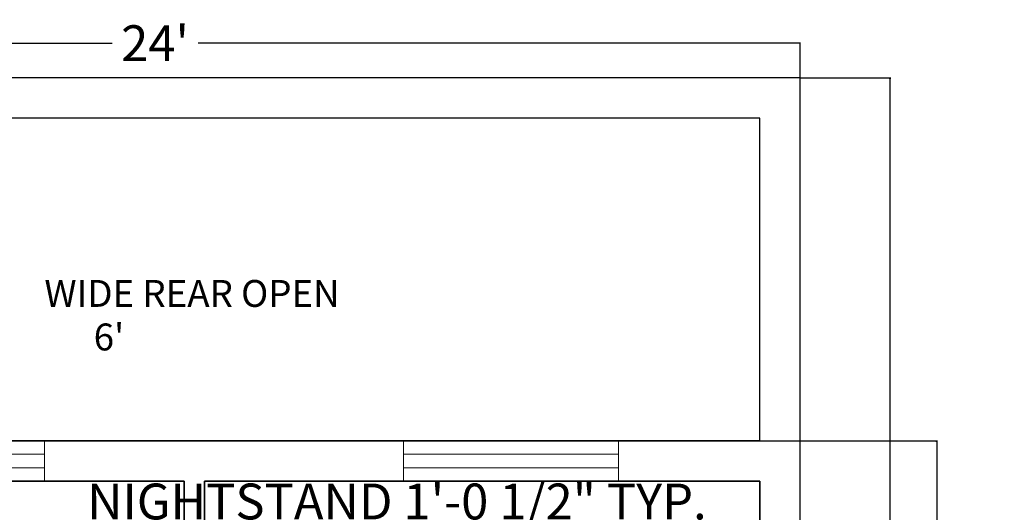
# Model space of a CAD drawing. Units: inches. Extents: x -11 to 443, y 65 to 743.
# Tile 10 of 10: x 158 to 378, y 610 to 720. Entities that reach past the tile are written whole.
import ezdxf

# ---------------------------------------------------------------- set-up
doc = ezdxf.new("R2010")
doc.units = ezdxf.units.IN
doc.header["$MEASUREMENT"] = 0
for name, color, linetype, lineweight in [('A-ANNO-DIMS', 2, 'Continuous', 18), ('A-AREA-IDEN', 2, 'Continuous', 18), ('A-GLAZ', 4, 'Continuous', 18), ('A-WALL', 7, 'Continuous', 35), ('A-WALL-SITE', 7, 'Continuous', 30), ('C-PROP', 3, 'Continuous', 30)]:
    doc.layers.add(name, color=color, linetype=linetype, lineweight=lineweight)
doc.styles.get("Standard").update_dxf_attribs({"font": 'italic8.shx'})
doc.dimstyles.get("Standard").update_dxf_attribs({"dimtxt": 8, "dimasz": 0.18, "dimexe": 0.18, "dimexo": 0.0625, "dimgap": 0.09, "dimtad": 0, "dimtih": 1, "dimtoh": 1, "dimzin": 0, "dimdsep": 46, "dimlunit": 3, "dimtxsty": 'Standard', "dimblk": 'CLOSEDBLANK', "dimcen": 0.09, "dimclrd": 6, "dimclre": 5, "dimclrt": 4, "dimadec": 0, "dimazin": 0, "dimtfac": 1, "dimtofl": 0, "dimtmove": 0, "dimatfit": 3, "dimfxl": 1, "dimtolj": 1, "dimtzin": 0, "dimarcsym": 0})

# ---------------------------------------------------------------- blocks, each defined once
blk = doc.blocks.new('_ClosedBlank')
at = {"color": 0, "linetype": 'ByBlock', "lineweight": -2}
for p, q in [((-1, 0.167), (0, 0)), ((-1, 0.167), (-1, -0.167)), ((0, 0), (-1, -0.167))]:
    blk.add_line(p, q, dxfattribs=at)
blk = doc.blocks.new('*D5')
at = {"layer": 'A-ANNO-DIMS', "color": 0, "lineweight": -2, "transparency": 16777216}
for p, q in [((44.21, 706.98), (44.21, 714.84)), ((44.39, 714.66), (178.6, 714.66)), ((332.03, 714.66), (197.82, 714.66)), ((332.21, 706.98), (332.21, 714.84))]:
    blk.add_line(p, q, dxfattribs=at)
at = {"layer": 'Defpoints', "color": 0, "lineweight": 100, "transparency": 16777216}
for p in [(332.21, 714.66), (44.21, 706.92), (332.21, 706.92)]:
    blk.add_point(p, dxfattribs=at)
at = {"layer": 'A-ANNO-DIMS', "color": 0, "lineweight": -2, "transparency": 16777216, "xscale": 0.18, "yscale": 0.18, "zscale": 0.18, "rotation": 180}
blk.add_blockref('_ClosedBlank', (44.21, 714.66), dxfattribs=at)
at = {"layer": 'A-ANNO-DIMS', "color": 0, "lineweight": -2, "transparency": 16777216, "xscale": 0.18, "yscale": 0.18, "zscale": 0.18}
blk.add_blockref('_ClosedBlank', (332.21, 714.66), dxfattribs=at)
at = {"layer": 'A-ANNO-DIMS', "color": 0, "transparency": 16777216, "insert": (188.21, 714.66), "char_height": 8, "attachment_point": 5}
blk.add_mtext("\\A1;24'", dxfattribs=at)
blk = doc.blocks.new('*D6')
at = {"layer": 'A-ANNO-DIMS', "color": 0, "lineweight": -2, "transparency": 16777216}
for p, q in [((332.27, 706.92), (352.4, 706.92)), ((352.22, 706.74), (352.22, 411.77)), ((352.22, 107.1), (352.22, 402.07)), ((332.27, 106.92), (352.4, 106.92))]:
    blk.add_line(p, q, dxfattribs=at)
at = {"layer": 'Defpoints', "color": 0, "lineweight": 100, "transparency": 16777216}
for p in [(332.21, 706.92), (332.21, 106.92), (352.22, 106.92)]:
    blk.add_point(p, dxfattribs=at)
at = {"layer": 'A-ANNO-DIMS', "color": 0, "lineweight": -2, "transparency": 16777216, "xscale": 0.18, "yscale": 0.18, "zscale": 0.18}
for p, rotation in [((352.22, 706.92), 90), ((352.22, 106.92), 270)]:
    blk.add_blockref('_ClosedBlank', p, dxfattribs=dict(at, rotation=rotation))
at = {"layer": 'A-ANNO-DIMS', "color": 0, "transparency": 16777216, "insert": (352.22, 406.92), "char_height": 8, "attachment_point": 5}
blk.add_mtext("\\A1;50'", dxfattribs=at)
blk = doc.blocks.new('WIN-48x9')
for p, q in [((0, 48), (0, 0)), ((9, 48), (0, 48)), ((3, 0), (3, 48)), ((6, 0), (6, 48)), ((9, 0), (9, 48)), ((0, 0), (9, 0))]:
    blk.add_line(p, q)
blk = doc.blocks.new('*D26')
at = {"layer": 'A-ANNO-DIMS', "color": 5, "lineweight": -2, "transparency": 16777216}
for p, q in [((133.01, 610.6), (133.01, 612.57)), ((145.34, 610.6), (145.34, 612.57))]:
    blk.add_line(p, q, dxfattribs=at)
at = {"layer": 'A-ANNO-DIMS', "color": 6, "lineweight": -2, "transparency": 16777216}
for p, q in [((133.19, 612.39), (145.16, 612.39)), ((145.34, 612.39), (145.52, 612.39))]:
    blk.add_line(p, q, dxfattribs=at)
at = {"layer": 'Defpoints', "color": 0, "lineweight": 100, "transparency": 16777216}
for p in [(145.34, 612.39), (133.01, 610.54), (145.34, 610.54)]:
    blk.add_point(p, dxfattribs=at)
at = {"layer": 'A-ANNO-DIMS', "color": 6, "lineweight": -2, "transparency": 16777216, "xscale": 0.18, "yscale": 0.18, "zscale": 0.18, "rotation": 180}
blk.add_blockref('_ClosedBlank', (133.01, 612.39), dxfattribs=at)
at = {"layer": 'A-ANNO-DIMS', "color": 6, "lineweight": -2, "transparency": 16777216, "xscale": 0.18, "yscale": 0.18, "zscale": 0.18}
blk.add_blockref('_ClosedBlank', (145.34, 612.39), dxfattribs=at)
at = {"layer": 'A-ANNO-DIMS', "color": 4, "transparency": 16777216, "insert": (242.18, 612.39), "char_height": 8, "attachment_point": 5}
blk.add_mtext('\\A1;NIGHTSTAND 1\'-0 1/2" TYP.', dxfattribs=at)
blk = doc.blocks.new('*D36')
at = {"layer": 'A-ANNO-DIMS', "color": 5, "lineweight": -2, "transparency": 16777216}
for p, q in [((323.27, 625.92), (362.85, 625.92)), ((323.27, 211.92), (362.85, 211.92))]:
    blk.add_line(p, q, dxfattribs=at)
at = {"layer": 'A-ANNO-DIMS', "color": 6, "lineweight": -2, "transparency": 16777216}
for p, q in [((362.67, 625.74), (362.67, 423.77)), ((362.67, 212.1), (362.67, 414.07))]:
    blk.add_line(p, q, dxfattribs=at)
at = {"layer": 'Defpoints', "color": 0, "lineweight": 100, "transparency": 16777216}
for p in [(323.21, 625.92), (362.67, 625.92), (323.21, 211.92)]:
    blk.add_point(p, dxfattribs=at)
at = {"layer": 'A-ANNO-DIMS', "color": 6, "lineweight": -2, "transparency": 16777216, "xscale": 0.18, "yscale": 0.18, "zscale": 0.18}
for p, rotation in [((362.67, 625.92), 90), ((362.67, 211.92), 270)]:
    blk.add_blockref('_ClosedBlank', p, dxfattribs=dict(at, rotation=rotation))
at = {"layer": 'A-ANNO-DIMS', "color": 4, "transparency": 16777216, "insert": (362.67, 418.92), "char_height": 8, "attachment_point": 5}
blk.add_mtext('\\A1;34\'-6"', dxfattribs=at)

msp = doc.modelspace()

# ---------------------------------------------------------------- linework, layer by layer
at = {"layer": 'A-WALL'}
for p, q in [((323.209, 625.92), (53.209, 625.92)), ((194.709, 616.92), (53.209, 616.92)), ((194.709, 616.92), (194.709, 522.42)), ((323.209, 616.92), (199.209, 616.92)), ((199.209, 616.92), (199.209, 522.42)), ((323.209, 522.42), (323.209, 616.92))]:
    msp.add_line(p, q, dxfattribs=at)
at = {"layer": 'A-WALL-SITE'}
for p, q in [((323.209, 697.92), (53.209, 697.92)), ((323.209, 625.92), (323.209, 697.92))]:
    msp.add_line(p, q, dxfattribs=at)
at = {"layer": 'C-PROP'}
msp.add_lwpolyline([(44.209, 106.92), (332.209, 106.92), (332.209, 706.92), (44.209, 706.92)], close=True, dxfattribs=at)

# ---------------------------------------------------------------- block references
at = {"layer": 'A-GLAZ', "rotation": 90.00000000000003}
for p in [(163.513, 616.92), (291.656, 616.92)]:
    msp.add_blockref('WIN-48x9', p, dxfattribs=at)

# ---------------------------------------------------------------- texts
at = {"layer": 'A-AREA-IDEN'}
for s, p in [('WIDE REAR OPEN', (163.503, 655.821)), ("      6'", (163.503, 646.107))]:
    msp.add_text(s, height=6, dxfattribs=at).set_placement(p)

# ---------------------------------------------------------------- dimensions: what is measured, and where the dimension line sits
at = {"layer": 'A-ANNO-DIMS'}
dim = msp.add_linear_dim(base=(332.209, 714.661), p1=(44.209, 706.92), p2=(332.209, 706.92), dimstyle='Standard', override={"dimclrd": 0, "dimclre": 0, "dimclrt": 0}, dxfattribs=at)
dim.commit()
dim.dimension.update_dxf_attribs({"geometry": '*D5', "text_midpoint": (188.209, 714.661)})
for base, p1, p2, override, picture, middle in [((352.221, 106.92), (332.209, 706.92), (332.209, 106.92), {"dimclrd": 0, "dimclre": 0, "dimclrt": 0}, '*D6', (352.221, 406.92)), ((362.669, 625.92), (323.209, 211.92), (323.209, 625.92), {"dimdec": 1, "dimlfac": 1, "dimrnd": 0, "dimzin": 1, "dimdsep": 46, "dimlunit": 4, "dimfrac": 2}, '*D36', (362.669, 418.92))]:
    dim = msp.add_linear_dim(base=base, p1=p1, p2=p2, angle=90, dimstyle='Standard', override=override, dxfattribs=at)
    dim.commit()
    dim.dimension.update_dxf_attribs({"geometry": picture, "text_midpoint": middle})
dim = msp.add_linear_dim(base=(145.337, 612.387), p1=(133.013, 610.539), p2=(145.337, 610.539), text='NIGHTSTAND <> TYP.', dimstyle='Standard', override={"dimdec": 1, "dimlfac": 1, "dimrnd": 0, "dimzin": 1, "dimdsep": 46, "dimlunit": 4, "dimfrac": 2}, dxfattribs=at)
dim.commit()
dim.dimension.update_dxf_attribs({"geometry": '*D26', "text_midpoint": (242.179, 612.387)})

doc.saveas('drawing.dxf')
